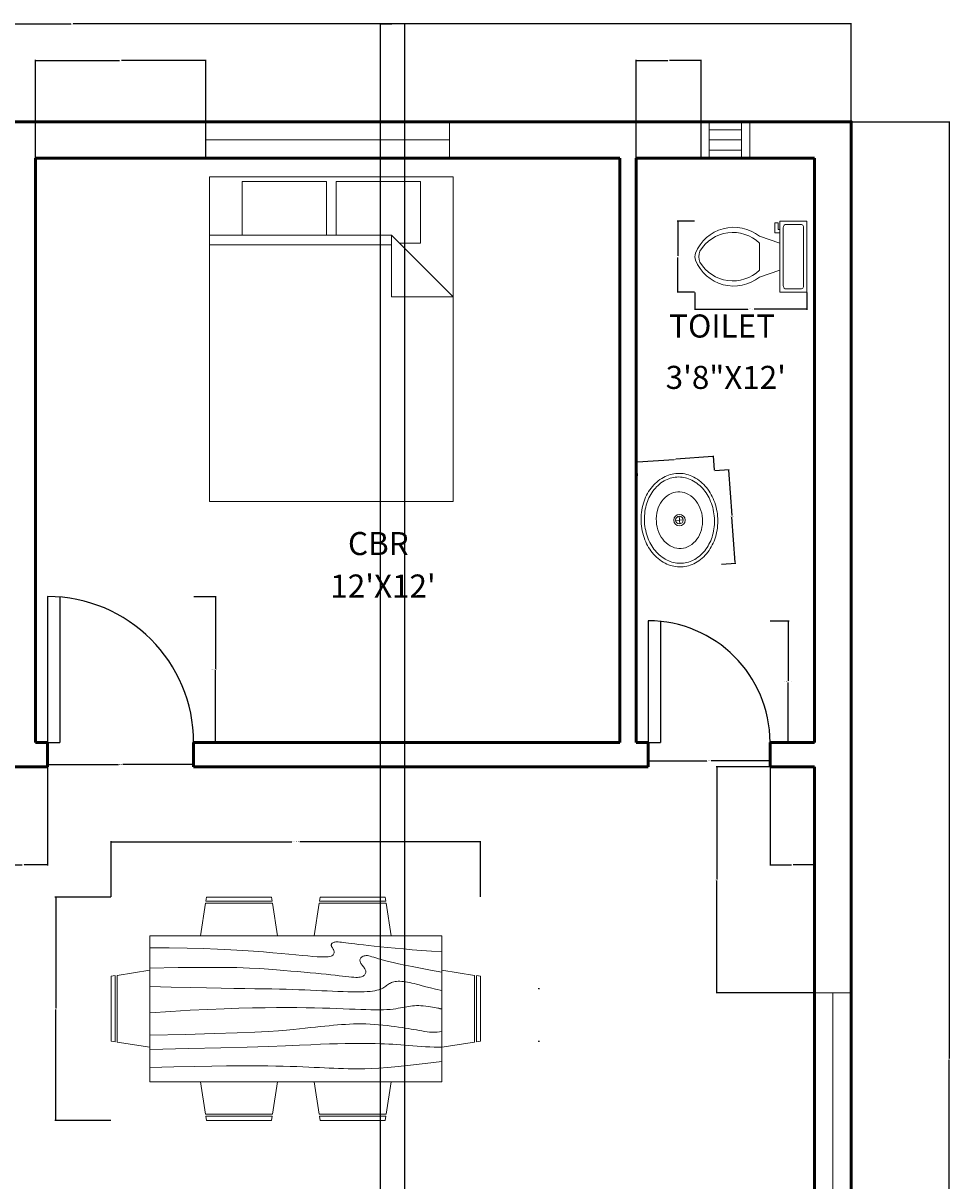
# Model space of a CAD drawing. Units: inches. Extents: x 66 to 499, y 601 to 1111.
# Tile 4 of 4: x 271 to 499, y 826 to 1111. Entities that reach past the tile are written whole.
import ezdxf

# ---------------------------------------------------------------- set-up
doc = ezdxf.new("R2010")
doc.units = ezdxf.units.IN
for name, color, linetype, lineweight in [('A-ANNO-DIMS', 2, 'Continuous', 18), ('A-AREA-IDEN', 7, 'Continuous', 18), ('A-DOOR', 3, 'Continuous', 25), ('A-FLOR-FIXT', 9, 'Continuous', 18), ('A-FURN', 8, 'Continuous', 18), ('A-GLAZ', 4, 'Continuous', 18), ('A-WALL', 7, 'Continuous', 50)]:
    doc.layers.add(name, color=color, linetype=linetype, lineweight=lineweight)
doc.styles.get("Standard").update_dxf_attribs({"font": 'arial.ttf'})
doc.dimstyles.get("Standard").update_dxf_attribs({"dimtxt": 0.18, "dimasz": 0.18, "dimexe": 0.18, "dimexo": 0.0625, "dimgap": 0.09, "dimtad": 0, "dimtih": 1, "dimtoh": 1, "dimdec": 4, "dimzin": 0, "dimdsep": 46, "dimtxsty": 'Standard', "dimcen": 0.09, "dimadec": 0, "dimazin": 0, "dimtfac": 1, "dimtdec": 4, "dimtofl": 0, "dimtmove": 0, "dimatfit": 3, "dimfxl": 1, "dimtolj": 1, "dimtzin": 0, "dimarcsym": 0})

# ---------------------------------------------------------------- blocks, each defined once
blk = doc.blocks.new('Dining Set - 36 x 72 in.')
for p, q in [((-22.2343, 26.00059), (-23.4847, 17.99762)), ((-22.2304, 26), (-5.7608, 26)), ((-22, 27.5), (-22.1562, 26.50042)), ((-5.8416, 26.5), (-22.1534, 26.5)), ((-22, 27.5), (-6, 27.5)), ((-5.8437, 26.49966), (-6, 27.5)), ((-4.5152, 17.99762), (-5.7655, 25.99926)), ((5.7657, 26.00059), (4.5153, 17.99762)), ((5.7696, 26), (22.2392, 26)), ((6, 27.5), (5.8438, 26.50042)), ((22.1584, 26.5), (5.8466, 26.5)), ((6, 27.5), (22, 27.5)), ((22.1563, 26.49966), (22, 27.5)), ((23.4848, 17.99762), (22.2345, 25.99926)), ((36, 18), (-36, 18)), ((-36, 18), (-36, -18)), ((36, -18), (36, 18)), ((-44.0006, 8.23428), (-35.9976, 9.48474)), ((44.0006, 8.23428), (35.9976, 9.48474)), ((-45.5, 8), (-44.5004, 8.15617)), ((-45.5, 8), (-45.5, -8)), ((-44.5, -8.15843), (-44.5, 8.15338)), ((-44, 8.23041), (-44, -8.23915)), ((44, 8.23041), (44, -8.23915)), ((44.5, -8.15843), (44.5, 8.15338)), ((45.5, 8), (44.5005, 8.15617)), ((45.5, 8), (45.5, -8)), ((-44.4997, -8.15631), (-45.5, -8)), ((-35.9976, -9.48476), (-43.9993, -8.2345)), ((35.9976, -9.48476), (43.9993, -8.2345)), ((44.4997, -8.15631), (45.5, -8)), ((-36, -18), (36, -18)), ((-22.2343, -26.0006), (-23.4847, -17.99762)), ((-4.5152, -17.99762), (-5.7655, -25.99928)), ((5.7657, -26.0006), (4.5153, -17.99762)), ((23.4848, -17.99762), (22.2345, -25.99928)), ((-22.2304, -26), (-5.7608, -26)), ((-22, -27.5), (-22.1562, -26.50044)), ((-5.8416, -26.5), (-22.1534, -26.5)), ((-22, -27.5), (-6, -27.5)), ((-5.8437, -26.49967), (-6, -27.5)), ((5.7696, -26), (22.2392, -26)), ((6, -27.5), (5.8438, -26.50044)), ((22.1584, -26.5), (5.8466, -26.5)), ((6, -27.5), (22, -27.5)), ((22.1563, -26.49967), (22, -27.5))]:
    blk.add_line(p, q)
for points in [[(-36, 15), (-31.1772, 14.97754), (-26.8079, 14.91406), (-22.8538, 14.81543), (-19.276, 14.6875), (-16.0362, 14.53613), (-13.0957, 14.36718), (-10.4159, 14.18652), (-7.9583, 14), (-5.6904, 13.81315), (-3.6035, 13.63021), (-1.6954, 13.45508), (0.0365, 13.29166), (1.5945, 13.14388), (2.9811, 13.01562), (4.1988, 12.9108), (5.25, 12.83333), (6.1393, 12.78613), (6.8802, 12.76823), (7.4883, 12.77767), (7.9792, 12.8125), (8.3685, 12.87077), (8.6719, 12.95052), (8.9049, 13.0498), (9.0833, 13.16666), (9.2205, 13.29899), (9.3216, 13.44401), (9.3895, 13.59879), (9.4271, 13.76041), (9.4373, 13.92594), (9.4232, 14.09245), (9.3875, 14.257), (9.3333, 14.41666), (9.2638, 14.56917), (9.1836, 14.71484), (9.0975, 14.85465), (9.0104, 14.98958), (8.9272, 15.1206), (8.8529, 15.2487), (8.7922, 15.37483), (8.75, 15.5), (8.7305, 15.62467), (8.7344, 15.74739), (8.7617, 15.86621), (8.8125, 15.97916), (8.8867, 16.08431), (8.9844, 16.17968), (9.1055, 16.26334), (9.25, 16.33333), (9.4189, 16.38802), (9.6172, 16.42708), (9.8506, 16.45052), (10.125, 16.45833), (10.4463, 16.45052), (10.8203, 16.42708), (11.2529, 16.38802), (11.75, 16.33333), (12.3184, 16.26318), (12.9694, 16.17838), (13.7151, 16.07991), (14.5677, 15.96875), (15.5395, 15.84586), (16.6426, 15.71224), (17.8893, 15.56884), (19.2917, 15.41666), (20.859, 15.25667), (22.5879, 15.08984), (24.4721, 14.91715), (26.5052, 14.73958), (28.6809, 14.5581), (30.9929, 14.3737), (33.4347, 14.18733), (36, 14)], [(-36, 10), (-28.9766, 10.14274), (-23.1725, 10.20442), (-18.4241, 10.19775), (-14.5677, 10.13541), (-11.4399, 10.03011), (-8.877, 9.89453), (-6.7154, 9.74137), (-4.7917, 9.58333), (-2.9698, 9.43082), (-1.2246, 9.28515), (0.4415, 9.14534), (2.026, 9.01041), (3.5266, 8.87939), (4.9408, 8.7513), (6.266, 8.62516), (7.5, 8.5), (8.6411, 8.37549), (9.6914, 8.2539), (10.6538, 8.13818), (11.5312, 8.03125), (12.3267, 7.93603), (13.043, 7.85547), (13.6831, 7.79248), (14.25, 7.75), (14.7471, 7.7303), (15.1797, 7.73307), (15.5537, 7.75732), (15.875, 7.80208), (16.1494, 7.86637), (16.3828, 7.94922), (16.5811, 8.04964), (16.75, 8.16666), (16.8944, 8.29915), (17.0143, 8.44531), (17.1089, 8.60319), (17.1771, 8.77083), (17.218, 8.94629), (17.2305, 9.1276), (17.2137, 9.31282), (17.1667, 9.5), (17.0895, 9.6875), (16.987, 9.875), (16.8649, 10.0625), (16.7292, 10.25), (16.5856, 10.4375), (16.4401, 10.625), (16.2985, 10.8125), (16.1667, 11), (16.05, 11.18733), (15.9518, 11.3737), (15.8752, 11.5581), (15.8229, 11.73958), (15.798, 11.91715), (15.8034, 12.08984), (15.842, 12.25667), (15.9167, 12.41666), (16.0295, 12.56836), (16.1784, 12.70833), (16.3605, 12.83268), (16.5729, 12.9375), (16.8127, 13.01888), (17.0768, 13.07291), (17.3625, 13.0957), (17.6667, 13.08333), (17.9894, 13.03312), (18.3418, 12.94726), (18.7382, 12.82918), (19.1927, 12.68229), (19.7195, 12.51001), (20.3327, 12.31575), (21.0465, 12.10294), (21.875, 11.875), (22.8357, 11.63354), (23.959, 11.37304), (25.2786, 11.08618), (26.8282, 10.76562), (28.6414, 10.40405), (30.752, 9.99414), (33.1936, 9.52856), (36, 9)], [(-36, 5.5), (-30.7157, 5.3348), (-26.069, 5.20963), (-21.9946, 5.11767), (-18.4271, 5.05208), (-15.3009, 5.00602), (-12.5508, 4.97265), (-10.1112, 4.94515), (-7.9167, 4.91666), (-5.909, 4.88167), (-4.0586, 4.83984), (-2.3429, 4.79215), (-0.7396, 4.73958), (0.7739, 4.6831), (2.22, 4.6237), (3.6213, 4.56233), (5, 4.5), (6.373, 4.43782), (7.7344, 4.3776), (9.0723, 4.32129), (10.375, 4.27083), (11.6309, 4.22819), (12.8281, 4.19531), (13.9551, 4.17415), (15, 4.16666), (15.954, 4.17448), (16.819, 4.19791), (17.6001, 4.23698), (18.3021, 4.29166), (18.9299, 4.36198), (19.4883, 4.44791), (19.9823, 4.54948), (20.4167, 4.66666), (20.7969, 4.79899), (21.1302, 4.94401), (21.4245, 5.09879), (21.6875, 5.26041), (21.9271, 5.42594), (22.1511, 5.59245), (22.3672, 5.757), (22.5834, 5.91666), (22.8065, 6.06868), (23.0404, 6.21093), (23.2879, 6.34147), (23.5521, 6.45833), (23.8358, 6.55957), (24.142, 6.64323), (24.4735, 6.70735), (24.8334, 6.75), (25.2235, 6.76969), (25.642, 6.76692), (26.0858, 6.74267), (26.5521, 6.69791), (27.0379, 6.63362), (27.5404, 6.55078), (28.0565, 6.45036), (28.5834, 6.33333), (29.1242, 6.19987), (29.7071, 6.04687), (30.3661, 5.87044), (31.1354, 5.66666), (32.0493, 5.43164), (33.142, 5.16146), (34.4475, 4.85221), (36, 4.5)], [(-36, -1), (-30.7915, -0.6591), (-26.0195, -0.38216), (-21.6519, -0.16284), (-17.6563, 0.00521), (-14.0005, 0.12833), (-10.6523, 0.21289), (-7.5796, 0.26522), (-4.75, 0.29166), (-2.134, 0.29793), (0.2878, 0.28711), (2.5317, 0.26163), (4.6146, 0.22396), (6.5529, 0.17651), (8.3633, 0.12174), (10.0623, 0.06209), (11.6667, 0), (13.1899, -0.06201), (14.6341, -0.1211), (15.9982, -0.17432), (17.2813, -0.21875), (18.4823, -0.25147), (19.6003, -0.26953), (20.6343, -0.27002), (21.5834, -0.25), (22.4481, -0.20768), (23.2357, -0.14584), (23.9549, -0.06836), (24.6146, 0.02083), (25.2235, 0.11784), (25.7904, 0.21875), (26.3241, 0.31966), (26.8334, 0.41666), (27.3265, 0.50618), (27.8099, 0.58593), (28.2894, 0.65397), (28.7709, 0.70833), (29.2601, 0.74707), (29.763, 0.76823), (30.2855, 0.76985), (30.8334, 0.75), (31.4088, 0.70784), (31.9994, 0.64713), (32.589, 0.57275), (33.1615, 0.48958), (33.7008, 0.4025), (34.1908, 0.3164), (34.6153, 0.23616), (34.9584, 0.16666), (35.2099, 0.11165), (35.3848, 0.07031), (35.504, 0.04069), (35.5886, 0.02083), (35.6594, 0.00879), (35.7377, 0.0026), (35.8442, 0.00032), (36, 0)], [(-36, -6.5), (-27.1843, -6.31267), (-20.084, -6.1263), (-14.469, -5.9419), (-10.1094, -5.76042), (-6.7752, -5.58285), (-4.2363, -5.41016), (-2.2629, -5.24333), (-0.625, -5.08334), (0.8708, -4.93099), (2.2715, -4.78646), (3.5872, -4.64974), (4.8281, -4.52084), (6.0046, -4.39974), (7.127, -4.28646), (8.2053, -4.18099), (9.25, -4.08334), (10.2705, -3.99382), (11.2734, -3.91407), (12.2647, -3.84603), (13.25, -3.79167), (14.2354, -3.75293), (15.2266, -3.73177), (16.2295, -3.73015), (17.25, -3.75), (18.2912, -3.79248), (19.3451, -3.85547), (20.4009, -3.93604), (21.4479, -4.03125), (22.4754, -4.13819), (23.4727, -4.25391), (24.4289, -4.37549), (25.3334, -4.5), (26.1785, -4.62492), (26.9694, -4.74935), (27.7145, -4.87281), (28.4219, -4.99479), (29.1, -5.11483), (29.7572, -5.23242), (30.4016, -5.34709), (31.0417, -5.45834), (31.6837, -5.56437), (32.3262, -5.65821), (32.9658, -5.73153), (33.599, -5.77604), (34.2224, -5.78345), (34.8327, -5.74545), (35.4264, -5.65373), (36, -5.5)], [(-36, -10), (-26.4022, -9.81299), (-18.4675, -9.62891), (-11.9839, -9.45069), (-6.7396, -9.28125), (-2.5226, -9.12354), (0.8789, -8.98047), (3.6769, -8.85498), (6.0833, -8.75), (8.2767, -8.66765), (10.3021, -8.60677), (12.1712, -8.56543), (13.8958, -8.54167), (15.4876, -8.53353), (16.9583, -8.53907), (18.3197, -8.55632), (19.5834, -8.58334), (20.7616, -8.61841), (21.8685, -8.66081), (22.9188, -8.71004), (23.9271, -8.76563), (24.9081, -8.82707), (25.8763, -8.89388), (26.8465, -8.96558), (27.8334, -9.04167), (28.8474, -9.12118), (29.8828, -9.20117), (30.93, -9.27824), (31.9792, -9.34896), (33.0205, -9.40991), (34.0443, -9.45768), (35.0407, -9.48885), (36, -9.5)], [(-36, -14.5), (-30.0881, -14.33513), (-25.0332, -14.21224), (-20.7312, -14.12647), (-17.0781, -14.07292), (-13.97, -14.04671), (-11.3027, -14.04297), (-8.9724, -14.05681), (-6.875, -14.08334), (-4.9224, -14.11833), (-3.0905, -14.16016), (-1.3709, -14.20785), (0.2448, -14.26042), (1.7647, -14.3169), (3.1973, -14.3763), (4.5507, -14.43767), (5.8333, -14.5), (7.0554, -14.5621), (8.235, -14.62175), (9.3922, -14.67652), (10.5469, -14.72396), (11.7192, -14.76164), (12.929, -14.78711), (14.1965, -14.79794), (15.5417, -14.79167), (16.9933, -14.76424), (18.6152, -14.70508), (20.4804, -14.60197), (22.6615, -14.44271), (25.2312, -14.21509), (28.2624, -13.9069), (31.8277, -13.50594), (36, -13)]]:
    blk.add_lwpolyline(points)
blk = doc.blocks.new('Sink - Oval top')
for p, q in [((-1, 0), (1, 0)), ((0, 1), (0, -1))]:
    blk.add_line(p, q)
for points in [[(-12.23, 0.39, 0.117634), (-11.46, -3.36, 0.104469), (-8.88, -6.8, 0.090016), (-5.08, -9.07, 0.08192), (-0.32, -10.02, 0.08192), (4.49, -9.38, 0.090016), (8.42, -7.36, 0.104469), (11.22, -4.09, 0.117634), (12.23, -0.39, 0.117634), (11.46, 3.36, 0.104469), (8.88, 6.8, 0.090016), (5.08, 9.07, 0.08192), (0.32, 10.02, 0.08192), (-4.49, 9.38, 0.090016), (-8.42, 7.36, 0.104469), (-11.22, 4.09, 0.117634)], [(-11.29, 0.16, 0.118622), (-10.52, -3.25, 0.104678), (-8.07, -6.36, 0.089562), (-4.54, -8.37, 0.081185), (-0.13, -9.15, 0.081185), (4.3, -8.49, 0.089562), (7.89, -6.58, 0.104678), (10.42, -3.55, 0.118622), (11.29, -0.16, 0.118622), (10.52, 3.25, 0.104678), (8.07, 6.36, 0.089562), (4.54, 8.37, 0.081185), (0.13, 9.15, 0.081185), (-4.3, 8.49, 0.089562), (-7.89, 6.58, 0.104678), (-10.42, 3.55, 0.118622)], [(-7.42, 0.08, 0.118283), (-6.91, -2.17, 0.104607), (-5.29, -4.21, 0.089718), (-2.97, -5.53, 0.081436), (-0.07, -6.04, 0.081436), (2.84, -5.59, 0.089718), (5.2, -4.33, 0.104607), (6.86, -2.32, 0.118283), (7.42, -0.08, 0.118283), (6.91, 2.17, 0.104607), (5.29, 4.21, 0.089718), (2.97, 5.53, 0.081436), (0.07, 6.04, 0.081436), (-2.84, 5.59, 0.089718), (-5.2, 4.33, 0.104607), (-6.86, 2.32, 0.118283)]]:
    blk.add_lwpolyline(points, format="xyb", close=True)
for radius in [1.5, 1]:
    blk.add_circle((0, 0), radius)
blk = doc.blocks.new('Toilet - top')
for p, q in [((9.5, -6), (9.5, -2)), ((-10, -8.5), (-8, -8.5)), ((-10, -9.5), (-10, -8.5)), ((-7, -9.5), (-10, -9.5)), ((-8, -8.5), (-8, -8)), ((-7, -8), (-7, -9.5)), ((-4, -8), (-6, -14)), ((4, -8), (6, -14)), ((4, -14), (-4, -14))]:
    blk.add_line(p, q)
blk.add_lwpolyline([(10.5, -8), (10.5, 0), (-10.5, 0), (-10.5, -8)], close=True)
for points in [[(-9.5, -2), (-9.5, -6)], [(8.5, -1), (-8.5, -1)], [(-8.5, -7), (8.5, -7)]]:
    blk.add_lwpolyline(points)
for centre, radius, start, end in [((-8.62, -1.88), 0.884, 81.8699, 188.1301), ((8.62, -1.88), 0.884, 351.8699, 98.1301), ((-8.62, -6.12), 0.884, 171.8699, 278.1301), ((8.62, -6.12), 0.884, 261.8699, 8.1301), ((3.52, -21.58), 12.17, 141.4691, 247.9714), ((4.2, -21.82), 11.33, 136.3677, 238.9468), ((-3.52, -21.58), 12.17, 292.0284, 38.5307), ((-4.2, -21.82), 11.33, 301.053, 43.6321), ((0, -27.88), 4, 245.7318, 294.2682), ((0, -29), 4, 254.8605, 285.1395)]:
    blk.add_arc(centre, radius, start, end)
blk = doc.blocks.new('Bed - Queen')
for p, q in [((0, -80.00003), (0, 0)), ((0, 0), (59.99999, 0)), ((59.99999, 0), (59.99999, -80.00003)), ((7.99999, -1.2), (28.79998, -1.2)), ((7.99999, -14.4), (7.99999, -1.2)), ((28.79998, -1.2), (28.79998, -14.4)), ((31.19999, -1.2), (51.99999, -1.2)), ((31.19999, -14.4), (31.19999, -1.2)), ((51.99999, -1.2), (51.99999, -16.4)), ((0, -14.4), (44.8, -14.4)), ((44.8, -16.8), (0, -16.8)), ((59.99999, -29.6), (44.8, -14.4)), ((44.8, -14.4), (44.8, -29.6)), ((51.99999, -16.4), (46.79936, -16.4)), ((44.8, -29.6), (59.99999, -29.6)), ((59.99999, -80.00003), (0, -80.00003))]:
    blk.add_line(p, q)
blk = doc.blocks.new('DOOR-SWING-36IN')
for p, q in [((0, 36), (0, 0)), ((3, 36), (3, 0)), ((0, 0), (3, 0))]:
    blk.add_line(p, q)
blk.add_arc((0, 0), 36, 0, 90)
blk = doc.blocks.new('DOOR-SWING-30IN')
for p, q in [((0, 30), (0, 0)), ((3, 30), (3, 0)), ((0, 0), (3, 0.01))]:
    blk.add_line(p, q)
blk.add_arc((0, 0), 30, 0.0977, 90)
blk = doc.blocks.new('WIN-60IN')
for p, q in [((60, 9), (0, 9)), ((0, 9), (0, 0)), ((60, 0), (60, 9)), ((0, 4.5), (60, 4.5)), ((0, 0), (60, 0))]:
    blk.add_line(p, q)
blk = doc.blocks.new('WIN-BATH-VENT-12IN')
for p, q in [((0, 12), (0, 0)), ((9, 12), (0, 12)), ((9, 0), (9, 12)), ((9, 10), (0, 10)), ((2, 10), (2, 2)), ((4.5, 10), (4.5, 2)), ((7, 2), (7, 10)), ((0, 2), (9, 2)), ((0, 0), (9, 0))]:
    blk.add_line(p, q)
blk = doc.blocks.new('*D18')
at = {"layer": 'A-ANNO-DIMS', "color": 0, "lineweight": -2, "transparency": 16777216}
for p, q in [((312.64, 970), (318.16, 970)), ((317.98, 969.82), (317.98, 952.19)), ((317.98, 934.18), (317.98, 951.82)), ((312.64, 934), (318.16, 934))]:
    blk.add_line(p, q, dxfattribs=at)
at = {"layer": 'A-ANNO-DIMS', "color": 0, "transparency": 16777216}
for points in [[(317.95, 969.82), (318.01, 969.82), (317.98, 970)], [(317.95, 934.18), (318.01, 934.18), (317.98, 934)]]:
    blk.add_solid(points, dxfattribs=at)
at = {"layer": 'Defpoints', "color": 0, "transparency": 16777216}
for p in [(312.58, 970), (317.98, 970), (312.58, 934)]:
    blk.add_point(p, dxfattribs=at)
at = {"layer": 'A-ANNO-DIMS', "color": 0, "transparency": 16777216, "insert": (317.98, 952), "char_height": 0.18, "attachment_point": 5}
blk.add_mtext('\\A1;BR DOOR 36 TYP.', dxfattribs=at)
blk = doc.blocks.new('*D19')
at = {"layer": 'A-ANNO-DIMS', "color": 0, "lineweight": -2, "transparency": 16777216}
for p, q in [((276.58, 933.94), (276.58, 928.42)), ((312.58, 933.94), (312.58, 928.42)), ((276.76, 928.6), (294.05, 928.6)), ((312.4, 928.6), (295.1, 928.6))]:
    blk.add_line(p, q, dxfattribs=at)
at = {"layer": 'A-ANNO-DIMS', "color": 0, "transparency": 16777216}
for points in [[(276.76, 928.63), (276.76, 928.57), (276.58, 928.6)], [(312.4, 928.63), (312.4, 928.57), (312.58, 928.6)]]:
    blk.add_solid(points, dxfattribs=at)
at = {"layer": 'Defpoints', "color": 0, "transparency": 16777216}
for p in [(276.58, 934), (312.58, 934), (312.58, 928.6)]:
    blk.add_point(p, dxfattribs=at)
at = {"layer": 'A-ANNO-DIMS', "color": 0, "transparency": 16777216, "insert": (294.58, 928.6), "char_height": 0.18, "attachment_point": 5}
blk.add_mtext('\\A1;36 TYP.', dxfattribs=at)
blk = doc.blocks.new('*D20')
at = {"layer": 'A-ANNO-DIMS', "color": 0, "lineweight": -2, "transparency": 16777216}
for p, q in [((440.96, 1001.04), (444.54, 1001.29)), ((444.37, 1001.1), (445.17, 989.92)), ((446, 978.38), (445.2, 989.56)), ((442.61, 977.96), (446.19, 978.22))]:
    blk.add_line(p, q, dxfattribs=at)
at = {"layer": 'A-ANNO-DIMS', "color": 0, "transparency": 16777216}
for points in [[(444.4, 1001.1), (444.34, 1001.1), (444.36, 1001.28)], [(446.03, 978.38), (445.97, 978.38), (446.01, 978.2)]]:
    blk.add_solid(points, dxfattribs=at)
at = {"layer": 'Defpoints', "color": 0, "transparency": 16777216}
for p in [(440.9, 1001.03), (442.55, 977.96), (446.01, 978.2)]:
    blk.add_point(p, dxfattribs=at)
at = {"layer": 'A-ANNO-DIMS', "color": 0, "transparency": 16777216, "insert": (445.19, 989.74), "char_height": 0.18, "attachment_point": 5}
blk.add_mtext('\\A1;BASIN 23', dxfattribs=at)
blk = doc.blocks.new('*D21')
at = {"layer": 'A-ANNO-DIMS', "color": 0, "lineweight": -2, "transparency": 16777216}
for p, q in [((440.47, 1004.48), (431.4, 1003.83)), ((440.89, 1001.09), (440.64, 1004.67)), ((421.97, 999.74), (421.71, 1003.32)), ((421.9, 1003.15), (430.98, 1003.8))]:
    blk.add_line(p, q, dxfattribs=at)
at = {"layer": 'A-ANNO-DIMS', "color": 0, "transparency": 16777216}
for points in [[(440.47, 1004.51), (440.47, 1004.45), (440.65, 1004.49)], [(421.9, 1003.18), (421.9, 1003.12), (421.72, 1003.14)]]:
    blk.add_solid(points, dxfattribs=at)
at = {"layer": 'Defpoints', "color": 0, "transparency": 16777216}
for p in [(440.65, 1004.49), (421.97, 999.68), (440.9, 1001.03)]:
    blk.add_point(p, dxfattribs=at)
at = {"layer": 'A-ANNO-DIMS', "color": 0, "transparency": 16777216, "insert": (431.19, 1003.82), "char_height": 0.18, "attachment_point": 5}
blk.add_mtext('\\A1;19', dxfattribs=at)
blk = doc.blocks.new('*D24')
at = {"layer": 'A-ANNO-DIMS', "color": 0, "lineweight": -2, "transparency": 16777216}
for p, q in [((436.05, 1044.9), (436.05, 1040.64)), ((463.68, 1044.9), (463.68, 1040.64)), ((436.23, 1040.82), (449.09, 1040.82)), ((463.5, 1040.82), (450.64, 1040.82))]:
    blk.add_line(p, q, dxfattribs=at)
at = {"layer": 'A-ANNO-DIMS', "color": 0, "transparency": 16777216}
for points in [[(436.23, 1040.85), (436.23, 1040.79), (436.05, 1040.82)], [(463.5, 1040.85), (463.5, 1040.79), (463.68, 1040.82)]]:
    blk.add_solid(points, dxfattribs=at)
at = {"layer": 'Defpoints', "color": 0, "transparency": 16777216}
for p in [(436.05, 1044.96), (463.68, 1044.96), (463.68, 1040.82)]:
    blk.add_point(p, dxfattribs=at)
at = {"layer": 'A-ANNO-DIMS', "color": 0, "transparency": 16777216, "insert": (449.86, 1040.82), "char_height": 0.18, "attachment_point": 5}
blk.add_mtext('\\A1;WC 28 TYP.', dxfattribs=at)
blk = doc.blocks.new('*D25')
at = {"layer": 'A-ANNO-DIMS', "color": 0, "lineweight": -2, "transparency": 16777216}
for p, q in [((435.98, 1062.52), (431.72, 1062.52)), ((431.9, 1062.34), (431.9, 1053.92)), ((431.9, 1045.14), (431.9, 1053.56)), ((435.98, 1044.96), (431.72, 1044.96))]:
    blk.add_line(p, q, dxfattribs=at)
at = {"layer": 'A-ANNO-DIMS', "color": 0, "transparency": 16777216}
for points in [[(431.87, 1062.34), (431.93, 1062.34), (431.9, 1062.52)], [(431.87, 1045.14), (431.93, 1045.14), (431.9, 1044.96)]]:
    blk.add_solid(points, dxfattribs=at)
at = {"layer": 'Defpoints', "color": 0, "transparency": 16777216}
for p in [(436.05, 1062.52), (431.9, 1044.96), (436.05, 1044.96)]:
    blk.add_point(p, dxfattribs=at)
at = {"layer": 'A-ANNO-DIMS', "color": 0, "transparency": 16777216, "insert": (431.9, 1053.74), "char_height": 0.18, "attachment_point": 5}
blk.add_mtext('\\A1;18 TYP.', dxfattribs=at)
blk = doc.blocks.new('*D26')
at = {"layer": 'A-ANNO-DIMS', "color": 0, "lineweight": -2, "transparency": 16777216}
for p, q in [((454.64, 964), (459.26, 964)), ((459.08, 963.82), (459.08, 949.19)), ((459.08, 934.18), (459.08, 948.82)), ((454.64, 934), (459.26, 934))]:
    blk.add_line(p, q, dxfattribs=at)
at = {"layer": 'A-ANNO-DIMS', "color": 0, "transparency": 16777216}
for points in [[(459.05, 963.82), (459.11, 963.82), (459.08, 964)], [(459.05, 934.18), (459.11, 934.18), (459.08, 934)]]:
    blk.add_solid(points, dxfattribs=at)
at = {"layer": 'Defpoints', "color": 0, "transparency": 16777216}
for p in [(454.58, 964), (459.08, 964), (454.58, 934)]:
    blk.add_point(p, dxfattribs=at)
at = {"layer": 'A-ANNO-DIMS', "color": 0, "transparency": 16777216, "insert": (459.08, 949), "char_height": 0.18, "attachment_point": 5}
blk.add_mtext('\\A1;WC DOOR 30 TYP.', dxfattribs=at)
blk = doc.blocks.new('*D27')
at = {"layer": 'A-ANNO-DIMS', "color": 0, "lineweight": -2, "transparency": 16777216}
for p, q in [((424.58, 933.94), (424.58, 929.32)), ((454.58, 933.94), (454.58, 929.32)), ((424.76, 929.5), (439.05, 929.5)), ((454.4, 929.5), (440.1, 929.5))]:
    blk.add_line(p, q, dxfattribs=at)
at = {"layer": 'A-ANNO-DIMS', "color": 0, "transparency": 16777216}
for points in [[(424.76, 929.53), (424.76, 929.47), (424.58, 929.5)], [(454.4, 929.53), (454.4, 929.47), (454.58, 929.5)]]:
    blk.add_solid(points, dxfattribs=at)
at = {"layer": 'Defpoints', "color": 0, "transparency": 16777216}
for p in [(424.58, 934), (454.58, 934), (454.58, 929.5)]:
    blk.add_point(p, dxfattribs=at)
at = {"layer": 'A-ANNO-DIMS', "color": 0, "transparency": 16777216, "insert": (439.58, 929.5), "char_height": 0.18, "attachment_point": 5}
blk.add_mtext('\\A1;30 TYP.', dxfattribs=at)
blk = doc.blocks.new('*D32')
at = {"layer": 'A-ANNO-DIMS', "color": 0, "lineweight": -2, "transparency": 16777216}
for p, q in [((292.25, 895.97), (292.25, 909.74)), ((292.43, 909.56), (336.8, 909.56)), ((383.07, 909.56), (338.7, 909.56)), ((383.25, 895.97), (383.25, 909.74))]:
    blk.add_line(p, q, dxfattribs=at)
at = {"layer": 'A-ANNO-DIMS', "color": 0, "transparency": 16777216}
for points in [[(292.43, 909.59), (292.43, 909.53), (292.25, 909.56)], [(383.07, 909.59), (383.07, 909.53), (383.25, 909.56)]]:
    blk.add_solid(points, dxfattribs=at)
at = {"layer": 'Defpoints', "color": 0, "transparency": 16777216}
for p in [(383.25, 909.56), (292.25, 895.91), (383.25, 895.91)]:
    blk.add_point(p, dxfattribs=at)
at = {"layer": 'A-ANNO-DIMS', "color": 0, "transparency": 16777216, "insert": (337.75, 909.56), "char_height": 0.18, "attachment_point": 5}
blk.add_mtext('\\A1;DINING SET 91', dxfattribs=at)
blk = doc.blocks.new('*D33')
at = {"layer": 'A-ANNO-DIMS', "color": 0, "lineweight": -2, "transparency": 16777216}
for p, q in [((292.19, 895.91), (278.42, 895.91)), ((278.6, 895.73), (278.6, 868.59)), ((278.6, 841.09), (278.6, 868.23)), ((292.19, 840.91), (278.42, 840.91))]:
    blk.add_line(p, q, dxfattribs=at)
at = {"layer": 'A-ANNO-DIMS', "color": 0, "transparency": 16777216}
for points in [[(278.57, 895.73), (278.63, 895.73), (278.6, 895.91)], [(278.57, 841.09), (278.63, 841.09), (278.6, 840.91)]]:
    blk.add_solid(points, dxfattribs=at)
at = {"layer": 'Defpoints', "color": 0, "transparency": 16777216}
for p in [(278.6, 895.91), (292.25, 895.91), (292.25, 840.91)]:
    blk.add_point(p, dxfattribs=at)
at = {"layer": 'A-ANNO-DIMS', "color": 0, "transparency": 16777216, "insert": (278.6, 868.41), "char_height": 0.18, "attachment_point": 5}
blk.add_mtext('\\A1;55', dxfattribs=at)
blk = doc.blocks.new('*D42')
at = {"layer": 'A-ANNO-DIMS', "color": 0, "lineweight": -2, "transparency": 16777216}
for p, q in [((90.58, 1087.07), (90.58, 1111.28)), ((90.76, 1111.1), (282.29, 1111.1)), ((474.4, 1111.1), (282.86, 1111.1)), ((474.58, 1087.07), (474.58, 1111.28))]:
    blk.add_line(p, q, dxfattribs=at)
at = {"layer": 'A-ANNO-DIMS', "color": 0, "transparency": 16777216}
for points in [[(90.76, 1111.13), (90.76, 1111.07), (90.58, 1111.1)], [(474.4, 1111.13), (474.4, 1111.07), (474.58, 1111.1)]]:
    blk.add_solid(points, dxfattribs=at)
at = {"layer": 'Defpoints', "color": 0, "transparency": 16777216}
for p in [(474.58, 1111.1), (90.58, 1087), (474.58, 1087)]:
    blk.add_point(p, dxfattribs=at)
at = {"layer": 'A-ANNO-DIMS', "color": 0, "transparency": 16777216, "insert": (282.58, 1111.1), "char_height": 0.18, "attachment_point": 5}
blk.add_mtext('\\A1;384', dxfattribs=at)
blk = doc.blocks.new('*D43')
at = {"layer": 'A-ANNO-DIMS', "color": 0, "lineweight": -2, "transparency": 16777216}
for p, q in [((474.64, 1087), (498.86, 1087)), ((498.68, 1086.82), (498.68, 856.19)), ((498.68, 625.18), (498.68, 855.82)), ((474.64, 625), (498.86, 625))]:
    blk.add_line(p, q, dxfattribs=at)
at = {"layer": 'A-ANNO-DIMS', "color": 0, "transparency": 16777216}
for points in [[(498.65, 1086.82), (498.71, 1086.82), (498.68, 1087)], [(498.65, 625.18), (498.71, 625.18), (498.68, 625)]]:
    blk.add_solid(points, dxfattribs=at)
at = {"layer": 'Defpoints', "color": 0, "transparency": 16777216}
for p in [(474.58, 1087), (498.68, 1087), (474.58, 625)]:
    blk.add_point(p, dxfattribs=at)
at = {"layer": 'A-ANNO-DIMS', "color": 0, "transparency": 16777216, "insert": (498.68, 856), "char_height": 0.18, "attachment_point": 5}
blk.add_mtext('\\A1;462', dxfattribs=at)
blk = doc.blocks.new('*D45')
at = {"layer": 'A-ANNO-DIMS', "color": 0, "lineweight": -2, "transparency": 16777216}
for p, q in [((273.58, 1078.07), (273.58, 1102.28)), ((273.76, 1102.1), (294.35, 1102.1)), ((315.4, 1102.1), (294.8, 1102.1)), ((315.58, 1078.07), (315.58, 1102.28))]:
    blk.add_line(p, q, dxfattribs=at)
at = {"layer": 'A-ANNO-DIMS', "color": 0, "transparency": 16777216}
for points in [[(273.76, 1102.13), (273.76, 1102.07), (273.58, 1102.1)], [(315.4, 1102.13), (315.4, 1102.07), (315.58, 1102.1)]]:
    blk.add_solid(points, dxfattribs=at)
at = {"layer": 'Defpoints', "color": 0, "transparency": 16777216}
for p in [(315.58, 1102.1), (273.58, 1078), (315.58, 1078)]:
    blk.add_point(p, dxfattribs=at)
at = {"layer": 'A-ANNO-DIMS', "color": 0, "transparency": 16777216, "insert": (294.58, 1102.1), "char_height": 0.18, "attachment_point": 5}
blk.add_mtext('\\A1;42', dxfattribs=at)
blk = doc.blocks.new('*D46')
at = {"layer": 'A-ANNO-DIMS', "color": 0, "lineweight": -2, "transparency": 16777216}
for p, q in [((421.58, 1078.07), (421.58, 1102.28)), ((421.76, 1102.1), (429.37, 1102.1)), ((437.4, 1102.1), (429.79, 1102.1)), ((437.58, 1078.07), (437.58, 1102.28))]:
    blk.add_line(p, q, dxfattribs=at)
at = {"layer": 'A-ANNO-DIMS', "color": 0, "transparency": 16777216}
for points in [[(421.76, 1102.13), (421.76, 1102.07), (421.58, 1102.1)], [(437.4, 1102.13), (437.4, 1102.07), (437.58, 1102.1)]]:
    blk.add_solid(points, dxfattribs=at)
at = {"layer": 'Defpoints', "color": 0, "transparency": 16777216}
for p in [(437.58, 1102.1), (421.58, 1078), (437.58, 1078)]:
    blk.add_point(p, dxfattribs=at)
at = {"layer": 'A-ANNO-DIMS', "color": 0, "transparency": 16777216, "insert": (429.58, 1102.1), "char_height": 0.18, "attachment_point": 5}
blk.add_mtext('\\A1;16', dxfattribs=at)
blk = doc.blocks.new('*D50')
at = {"layer": 'A-ANNO-DIMS', "color": 0, "lineweight": -2, "transparency": 16777216}
for p, q in [((465.51, 928), (441.3, 928.01)), ((441.48, 927.83), (441.47, 900.37)), ((441.47, 872.55), (441.47, 900.01)), ((465.5, 872.37), (441.29, 872.37))]:
    blk.add_line(p, q, dxfattribs=at)
at = {"layer": 'A-ANNO-DIMS', "color": 0, "transparency": 16777216}
for points in [[(441.45, 927.83), (441.51, 927.83), (441.48, 928.01)], [(441.44, 872.55), (441.5, 872.55), (441.47, 872.37)]]:
    blk.add_solid(points, dxfattribs=at)
at = {"layer": 'Defpoints', "color": 0, "transparency": 16777216}
for p in [(441.48, 928.01), (465.58, 928), (465.57, 872.37)]:
    blk.add_point(p, dxfattribs=at)
at = {"layer": 'A-ANNO-DIMS', "color": 0, "transparency": 16777216, "insert": (441.47, 900.19), "char_height": 0.18, "attachment_point": 5}
blk.add_mtext('\\A1;55.64', dxfattribs=at)
blk = doc.blocks.new('*D55')
at = {"layer": 'A-ANNO-DIMS', "color": 0, "lineweight": -2, "transparency": 16777216}
for p, q in [((358.58, 659.57), (358.58, 1111.28)), ((358.76, 1111.1), (361.43, 1111.1)), ((364.4, 1111.1), (361.73, 1111.1)), ((364.58, 659.57), (364.58, 1111.28))]:
    blk.add_line(p, q, dxfattribs=at)
at = {"layer": 'A-ANNO-DIMS', "color": 0, "transparency": 16777216}
for points in [[(358.76, 1111.13), (358.76, 1111.07), (358.58, 1111.1)], [(364.4, 1111.13), (364.4, 1111.07), (364.58, 1111.1)]]:
    blk.add_solid(points, dxfattribs=at)
at = {"layer": 'Defpoints', "color": 0, "transparency": 16777216}
for p in [(364.58, 1111.1), (358.58, 659.5), (364.58, 659.5)]:
    blk.add_point(p, dxfattribs=at)
at = {"layer": 'A-ANNO-DIMS', "color": 0, "transparency": 16777216, "insert": (361.58, 1111.1), "char_height": 0.18, "attachment_point": 5}
blk.add_mtext('\\A1;6', dxfattribs=at)
blk = doc.blocks.new('*D58')
at = {"layer": 'A-ANNO-DIMS', "color": 0, "lineweight": -2, "transparency": 16777216}
for p, q in [((264.58, 927.94), (264.58, 903.72)), ((276.58, 927.94), (276.58, 903.72)), ((264.76, 903.9), (270.37, 903.9)), ((276.4, 903.9), (270.79, 903.9))]:
    blk.add_line(p, q, dxfattribs=at)
at = {"layer": 'A-ANNO-DIMS', "color": 0, "transparency": 16777216}
for points in [[(264.76, 903.93), (264.76, 903.87), (264.58, 903.9)], [(276.4, 903.93), (276.4, 903.87), (276.58, 903.9)]]:
    blk.add_solid(points, dxfattribs=at)
at = {"layer": 'Defpoints', "color": 0, "transparency": 16777216}
for p in [(264.58, 928), (276.58, 928), (264.58, 903.9)]:
    blk.add_point(p, dxfattribs=at)
at = {"layer": 'A-ANNO-DIMS', "color": 0, "transparency": 16777216, "insert": (270.58, 903.9), "char_height": 0.18, "attachment_point": 5}
blk.add_mtext('\\A1;12', dxfattribs=at)
blk = doc.blocks.new('*D63')
at = {"layer": 'A-ANNO-DIMS', "color": 0, "lineweight": -2, "transparency": 16777216}
for p, q in [((454.58, 927.94), (454.58, 903.72)), ((465.58, 927.94), (465.58, 903.72)), ((454.76, 903.9), (459.88, 903.9)), ((465.4, 903.9), (460.27, 903.9))]:
    blk.add_line(p, q, dxfattribs=at)
at = {"layer": 'A-ANNO-DIMS', "color": 0, "transparency": 16777216}
for points in [[(454.76, 903.93), (454.76, 903.87), (454.58, 903.9)], [(465.4, 903.93), (465.4, 903.87), (465.58, 903.9)]]:
    blk.add_solid(points, dxfattribs=at)
at = {"layer": 'Defpoints', "color": 0, "transparency": 16777216}
for p in [(454.58, 928), (465.58, 928), (454.58, 903.9)]:
    blk.add_point(p, dxfattribs=at)
at = {"layer": 'A-ANNO-DIMS', "color": 0, "transparency": 16777216, "insert": (460.08, 903.9), "char_height": 0.18, "attachment_point": 5}
blk.add_mtext('\\A1;11', dxfattribs=at)
blk = doc.blocks.new('*D68')
at = {"layer": 'A-ANNO-DIMS', "color": 0, "lineweight": -2, "transparency": 16777216}
for p, q in [((397.57, 873.38), (397.75, 873.38)), ((397.66, 873.29), (397.66, 873.47)), ((397.66, 679.46), (397.66, 752)), ((397.84, 679.46), (397.66, 679.46))]:
    blk.add_line(p, q, dxfattribs=at)
at = {"layer": 'A-ANNO-DIMS', "color": 0, "transparency": 16777216}
blk.add_solid([(397.69, 752), (397.63, 752), (397.66, 752.18)], dxfattribs=at)
at = {"layer": 'Defpoints', "color": 0, "transparency": 16777216}
for p in [(397.66, 873.38), (397.66, 752.18)]:
    blk.add_point(p, dxfattribs=at)
at = {"layer": 'A-ANNO-DIMS', "color": 0, "transparency": 16777216, "insert": (398.32, 679.46), "char_height": 0.18, "attachment_point": 5}
blk.add_mtext('\\A1;R121.2', dxfattribs=at)
blk = doc.blocks.new('*D69')
at = {"layer": 'A-ANNO-DIMS', "color": 0, "lineweight": -2, "transparency": 16777216}
for p, q in [((397.57, 860.43), (397.75, 860.43)), ((397.66, 860.34), (397.66, 860.52)), ((397.66, 677.63), (397.66, 746)), ((397.84, 677.63), (397.66, 677.63))]:
    blk.add_line(p, q, dxfattribs=at)
at = {"layer": 'A-ANNO-DIMS', "color": 0, "transparency": 16777216}
blk.add_solid([(397.69, 746), (397.63, 746), (397.66, 746.18)], dxfattribs=at)
at = {"layer": 'Defpoints', "color": 0, "transparency": 16777216}
for p in [(397.66, 860.43), (397.66, 746.18)]:
    blk.add_point(p, dxfattribs=at)
at = {"layer": 'A-ANNO-DIMS', "color": 0, "transparency": 16777216, "insert": (398.39, 677.63), "char_height": 0.18, "attachment_point": 5}
blk.add_mtext('\\A1;R114.25', dxfattribs=at)

msp = doc.modelspace()

# ---------------------------------------------------------------- linework, layer by layer
at = {"layer": 'A-WALL'}
for p, q in [((273.5757, 1078.0042), (273.5757, 934.0042)), ((417.5757, 1078.0042), (273.5757, 1078.0042)), ((417.5757, 1078.0042), (417.5757, 934.0042)), ((465.5757, 1078.0042), (421.5757, 1078.0042)), ((421.5757, 1078.0042), (421.5757, 934.0042)), ((465.5757, 934.0042), (465.5757, 1078.0042)), ((276.5757, 934.0042), (273.5757, 934.0042)), ((276.5757, 934.0042), (276.5757, 928.0042)), ((312.5757, 934.0042), (312.5757, 928.0042)), ((417.5757, 934.0042), (312.5757, 934.0042)), ((424.5757, 934.0042), (421.5757, 934.0042)), ((424.5757, 934.0042), (424.5757, 928.0042)), ((465.5757, 934.0042), (454.5757, 934.0042)), ((454.5757, 934.0042), (454.5757, 928.0042)), ((267.5757, 928.0042), (273.5757, 928.0042)), ((276.5757, 928.0042), (273.5757, 928.0042)), ((424.5757, 928.0042), (312.5757, 928.0042)), ((465.5757, 928.0042), (454.5757, 928.0042)), ((465.5757, 742.0042), (465.5757, 928.0042))]:
    msp.add_line(p, q, dxfattribs=at)
msp.add_lwpolyline([(90.5757, 625.0042), (474.5757, 625.0042), (474.5757, 1087.0042), (90.5757, 1087.0042)], close=True, dxfattribs=at)

# ---------------------------------------------------------------- block references
at = {"layer": 'A-DOOR'}
for name, p in [('DOOR-SWING-36IN', (276.5757, 934.0042)), ('DOOR-SWING-30IN', (424.5757, 934.0042))]:
    msp.add_blockref(name, p, dxfattribs=at)
at = {"layer": 'A-FLOR-FIXT'}
for name, p, xscale, yscale, zscale, rotation in [('Toilet - top', (463.6816, 1053.7413), 0.8362564653676912, 0.8362564653676912, 0.8362564653676912, 270), ('Sink - Oval top', (432.2598, 988.8171), 0.9423771683571505, 0.9423771683571505, 0.9423771683571505, 274.0895995731086)]:
    msp.add_blockref(name, p, dxfattribs=dict(at, xscale=xscale, yscale=yscale, zscale=zscale, rotation=rotation))
at = {"layer": 'A-FURN'}
for name, p in [('Bed - Queen', (316.4991, 1073.4386)), ('Dining Set - 36 x 72 in.', (337.7521, 868.411))]:
    msp.add_blockref(name, p, dxfattribs=at)
at = {"layer": 'A-GLAZ'}
msp.add_blockref('WIN-60IN', (315.5757, 1078.0042), dxfattribs=at)
for name, p, rotation in [('WIN-BATH-VENT-12IN', (449.5757, 1078.0042), 89.99999999999909), ('WIN-60IN', (465.5667, 872.3672), 270.0000000000001)]:
    msp.add_blockref(name, p, dxfattribs=dict(at, rotation=rotation))

# ---------------------------------------------------------------- texts
at = {"layer": 'A-AREA-IDEN', "char_height": 5.6821, "attachment_point": 1}
for s, insert in [('TOILET', (429.7367, 1039.4919)), ('3\'8"X12\'', (428.8629, 1026.8342)), ('CBR', (350.5959, 985.8882)), ("12'X12'", (346.2581, 975.4196))]:
    msp.add_mtext_dynamic_manual_height_columns(s, width=58.656418, gutter_width=28.4105, heights=[0], dxfattribs=dict(at, insert=insert))

# ---------------------------------------------------------------- dimensions: what is measured, and where the dimension line sits
at = {"layer": 'A-ANNO-DIMS'}
for base, p1, p2, picture, middle in [((474.5757, 1111.1042), (90.5757, 1087.0042), (474.5757, 1087.0042), '*D42', (282.5757, 1111.1042)), ((364.5757, 1111.1042), (358.5757, 659.5042), (364.5757, 659.5042), '*D55', (361.5757, 1111.1042))]:
    dim = msp.add_linear_dim(base=base, p1=p1, p2=p2, dimstyle='Standard', override={"dimdec": 0, "dimlfac": 1, "dimrnd": 0, "dimzin": 0, "dimdsep": 46, "dimlunit": 2}, dxfattribs=at)
    dim.commit()
    dim.dimension.update_dxf_attribs({"geometry": picture, "text_midpoint": middle})
for base, p1, p2, angle, override, picture, middle in [((315.5757, 1102.1042), (273.5757, 1078.0042), (315.5757, 1078.0042), 0, {"dimdec": 0, "dimlfac": 1, "dimrnd": 0, "dimzin": 0, "dimdsep": 46, "dimlunit": 2}, '*D45', (294.5757, 1102.1042)), ((437.5757, 1102.1042), (421.5757, 1078.0042), (437.5757, 1078.0042), 0, {"dimdec": 0, "dimlfac": 1, "dimrnd": 0, "dimzin": 0, "dimdsep": 46, "dimlunit": 2}, '*D46', (429.5757, 1102.1042)), ((498.6757, 1087.0042), (474.5757, 625.0042), (474.5757, 1087.0042), 90, {"dimdec": 0, "dimlfac": 1, "dimrnd": 0, "dimzin": 0, "dimdsep": 46, "dimlunit": 2}, '*D43', (498.6757, 856.0042)), ((440.6512, 1004.494), (421.9708, 999.6791), (440.8987, 1001.0324), 4.0896, {"dimdec": 0, "dimlfac": 1, "dimrnd": 0, "dimzin": 0, "dimdsep": 46, "dimlunit": 2}, '*D21', (431.1873, 1003.8173)), ((264.5757, 903.9042), (276.5757, 928.0042), (264.5757, 928.0042), 180, {"dimdec": 0, "dimlfac": 1, "dimrnd": 0, "dimzin": 0, "dimdsep": 46, "dimlunit": 2}, '*D58', (270.5757, 903.9042)), ((441.4757, 928.0081), (465.5667, 872.3672), (465.5757, 928.0042), 89.990752, {"dimdec": 2, "dimlfac": 1, "dimrnd": 0, "dimzin": 0, "dimdsep": 46, "dimlunit": 2}, '*D50', (441.4712, 900.1896)), ((454.5757, 903.9042), (465.5757, 928.0042), (454.5757, 928.0042), 180, {"dimdec": 0, "dimlfac": 1, "dimrnd": 0, "dimzin": 0, "dimdsep": 46, "dimlunit": 2}, '*D63', (460.0757, 903.9042)), ((278.6021, 895.911), (292.2521, 840.911), (292.2521, 895.911), 90, {"dimdec": 0, "dimlfac": 1, "dimrnd": 0, "dimzin": 0, "dimdsep": 46, "dimlunit": 2}, '*D33', (278.6021, 868.411))]:
    dim = msp.add_linear_dim(base=base, p1=p1, p2=p2, angle=angle, dimstyle='Standard', override=override, dxfattribs=at)
    dim.commit()
    dim.dimension.update_dxf_attribs({"geometry": picture, "text_midpoint": middle})
for base, p1, p2, angle, text, picture, middle in [((431.9012, 1044.9606), (436.0465, 1062.522), (436.0465, 1044.9606), 270, '<> TYP.', '*D25', (431.9012, 1053.7413)), ((446.0103, 978.2026), (440.8987, 1001.0324), (442.5487, 977.9551), 274.0896, 'BASIN <>', '*D20', (445.1853, 989.7412)), ((317.9757, 970.0042), (312.5757, 934.0042), (312.5757, 970.0042), 90, 'BR DOOR <> TYP.', '*D18', (317.9757, 952.0042)), ((459.0756, 964.0042), (454.5756, 934.0042), (454.5756, 964.0042), 90, 'WC DOOR <> TYP.', '*D26', (459.0756, 949.0042))]:
    dim = msp.add_linear_dim(base=base, p1=p1, p2=p2, angle=angle, text=text, dimstyle='Standard', override={"dimdec": 0, "dimlfac": 1, "dimrnd": 0, "dimzin": 0, "dimdsep": 46, "dimlunit": 2}, dxfattribs=at)
    dim.commit()
    dim.dimension.update_dxf_attribs({"geometry": picture, "text_midpoint": middle})
for base, p1, p2, text, picture, middle in [((463.6816, 1040.8153), (436.0465, 1044.9606), (463.6816, 1044.9606), 'WC <> TYP.', '*D24', (449.864, 1040.8153)), ((312.5757, 928.6042), (276.5757, 934.0042), (312.5757, 934.0042), '<> TYP.', '*D19', (294.5757, 928.6042)), ((454.5756, 929.5042), (424.5757, 934.0042), (454.5756, 934.0042), '<> TYP.', '*D27', (439.5757, 929.5042)), ((383.2521, 909.561), (292.2521, 895.911), (383.2521, 895.911), 'DINING SET <>', '*D32', (337.7521, 909.561))]:
    dim = msp.add_linear_dim(base=base, p1=p1, p2=p2, text=text, dimstyle='Standard', override={"dimdec": 0, "dimlfac": 1, "dimrnd": 0, "dimzin": 0, "dimdsep": 46, "dimlunit": 2}, dxfattribs=at)
    dim.commit()
    dim.dimension.update_dxf_attribs({"geometry": picture, "text_midpoint": middle})
for center, mpoint, override, picture, middle in [((397.6569, 873.3791), (397.657, 752.1823), {"dimdec": 1, "dimlfac": 1, "dimrnd": 0, "dimzin": 0, "dimdsep": 46, "dimlunit": 2}, '*D68', (398.316, 679.4643)), ((397.6569, 860.4323), (397.657, 746.1823), {"dimdec": 2, "dimlfac": 1, "dimrnd": 0, "dimzin": 0, "dimdsep": 46, "dimlunit": 2}, '*D69', (398.3875, 677.6323))]:
    dim = msp.add_radius_dim(center=center, mpoint=mpoint, dimstyle='Standard', override=override, dxfattribs=at)
    dim.commit()
    dim.dimension.update_dxf_attribs({"geometry": picture, "text_midpoint": middle, "dimtype": 164})

doc.saveas('drawing.dxf')
